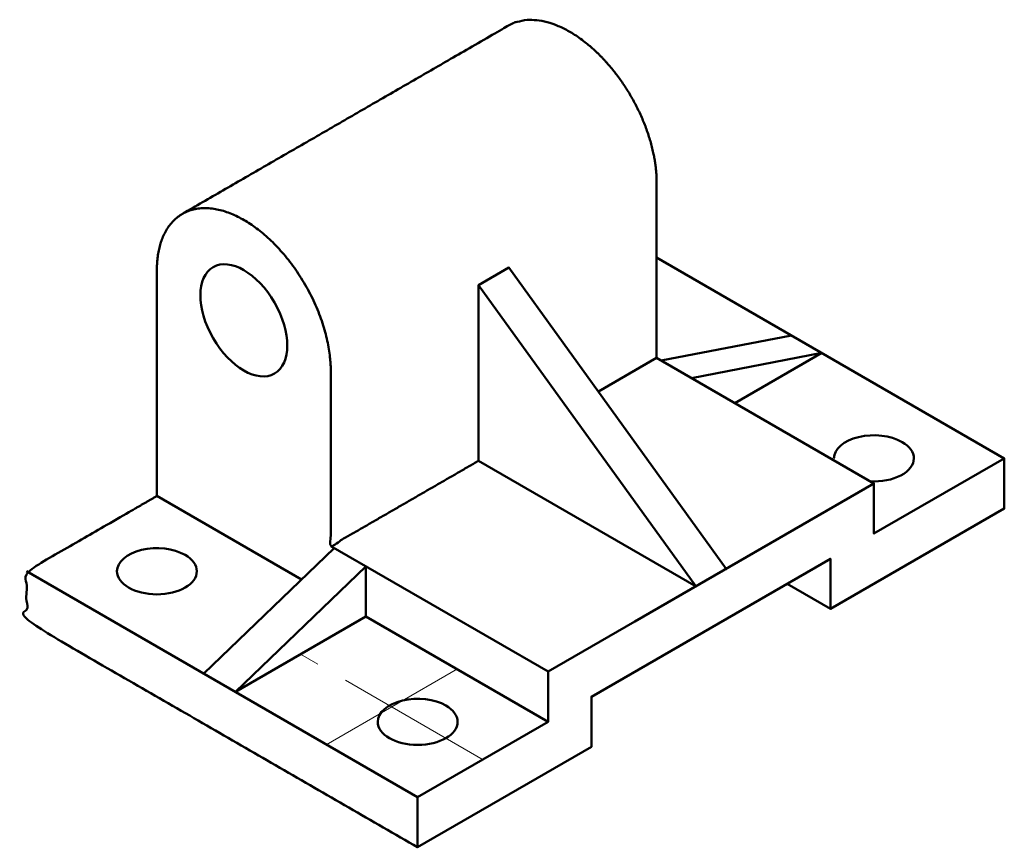
# Model space of a CAD drawing. Units: millimetres. Extents: x -1 to 195, y 18 to 183.
import ezdxf

# ---------------------------------------------------------------- set-up
doc = ezdxf.new("R2010")
doc.units = ezdxf.units.MM
doc.header["$MEASUREMENT"] = 0
doc.linetypes.add('CENTER', pattern=[50.8, 31.75, -6.35, 6.35, -6.35])
doc.layers.add('M-CNTR', color=1, linetype='CENTER', lineweight=18)
doc.layers.add('M-OUTL', color=7, linetype='Continuous', lineweight=50)

# ---------------------------------------------------------------- blocks, each defined once
blk = doc.blocks.new('*U1')
at = {"layer": 'M-CNTR', "color": 0, "transparency": 16777216}
blk.add_line((13.09, 7.56), (-13.09, -7.56), dxfattribs=at)

msp = doc.modelspace()

# ---------------------------------------------------------------- linework, layer by layer
at = {"layer": 'M-CNTR'}
msp.add_line((91.08, 35.14), (54.67, 56.16), dxfattribs=at)
at = {"layer": 'M-OUTL'}
for p, q in [((152.47, 119.7), (126.49, 114.7)), ((158.53, 116.2), (132.55, 111.2)), ((141.21, 106.2), (158.53, 116.2)), ((54.85, 71.06), (26.03, 87.7)), ((35.37, 52.31), (61.35, 77.31)), ((160.26, 65.2), (151.6, 70.2)), ((103.97, 42.7), (77.99, 27.7))]:
    msp.add_line(p, q, dxfattribs=at)
for points in [[(114, 108.5), (125.62, 115.2), (168.92, 90.2), (168.92, 80.2), (194.9, 95.2), (125.62, 135.2)], [(133.41, 69.7), (90.11, 129.7), (96.17, 133.2), (139.48, 73.2), (139.58, 73.14)], [(133.52, 69.64), (90.11, 94.7), (90.11, 129.7)], [(194.9, 95.2), (194.9, 85.2), (160.26, 65.2), (160.26, 75.2), (112.63, 47.7), (112.63, 37.7), (77.99, 17.7), (77.99, 27.7), (0.05, 72.7)], [(168.92, 90.2), (121.29, 62.7), (103.97, 52.7)], [(67.66, 63.66), (103.97, 42.7), (103.97, 52.7), (60.67, 77.7)]]:
    msp.add_lwpolyline(points, dxfattribs=at)
msp.add_lwpolyline([(67.66, 73.66), (67.66, 63.66), (41.68, 48.66)], close=True, dxfattribs=at)
msp.add_ellipse((43.35, 122.7), major_axis=(6.12, -10.61), ratio=0.57735, dxfattribs=at)
for centre, start_param, end_param in [((168.92, 95.2), 0.785398, 3.141593), ((168.92, 95.2), 0, 0.785398), ((168.92, 95.2), 4.620151, 6.283185), ((26.03, 72.7), 0.785398, 3.141593), ((26.03, 72.7), 0, 0.785398), ((26.03, 72.7), 3.141593, 6.283185), ((77.99, 42.7), 0.785398, 3.141593), ((77.99, 42.7), 0, 0.785398), ((77.99, 42.7), 3.141593, 6.283185)]:
    msp.add_ellipse(centre, major_axis=(7.96, 0), ratio=0.57735, start_param=start_param, end_param=end_param, dxfattribs=at)
for points, weights, knots in [([(125.62, 115.2), (125.62, 132.7), (125.62, 150.2), (125.62, 163.56), (114.93, 174.85), (104.23, 186.14), (96.05, 181.41), (63.58, 162.66), (31.1, 143.91)], [1, 1, 1, 0.831469612303, 1, 0.831469612303, 1, 1, 1], [0, 0, 0, 1, 1, 2.178097, 2.178097, 3.356194, 3.356194, 4.356194, 4.356194, 4.356194]), ([(90.11, 94.7), (75.39, 86.2), (60.67, 77.7), (60.67, 95.2), (60.67, 112.7), (60.67, 132.7), (43.35, 142.7), (26.03, 152.7), (26.03, 132.7), (26.03, 115.2), (26.03, 97.7), (26.03, 92.7), (26.03, 87.7), (13.04, 80.2), (0.05, 72.7), (0.05, 67.7), (0.05, 62.7), (39.02, 40.2), (77.99, 17.7)], [1, 1, 1, 1, 1, 0.707106781187, 1, 0.707106781187, 1, 1, 1, 1, 1, 1, 1, 1, 1, 1, 1], [0, 0, 0, 1, 1, 2, 2, 3.570796, 3.570796, 5.141593, 5.141593, 6.141593, 6.141593, 7.141593, 7.141593, 8.141593, 8.141593, 9.141593, 9.141593, 10.141593, 10.141593, 10.141593])]:
    msp.add_rational_spline(points, weights, degree=2, knots=knots, dxfattribs=at)

# ---------------------------------------------------------------- block references
at = {"layer": 'M-CNTR'}
msp.add_blockref('*U1', (72.82, 45.68), dxfattribs=at)

doc.saveas('drawing.dxf')
